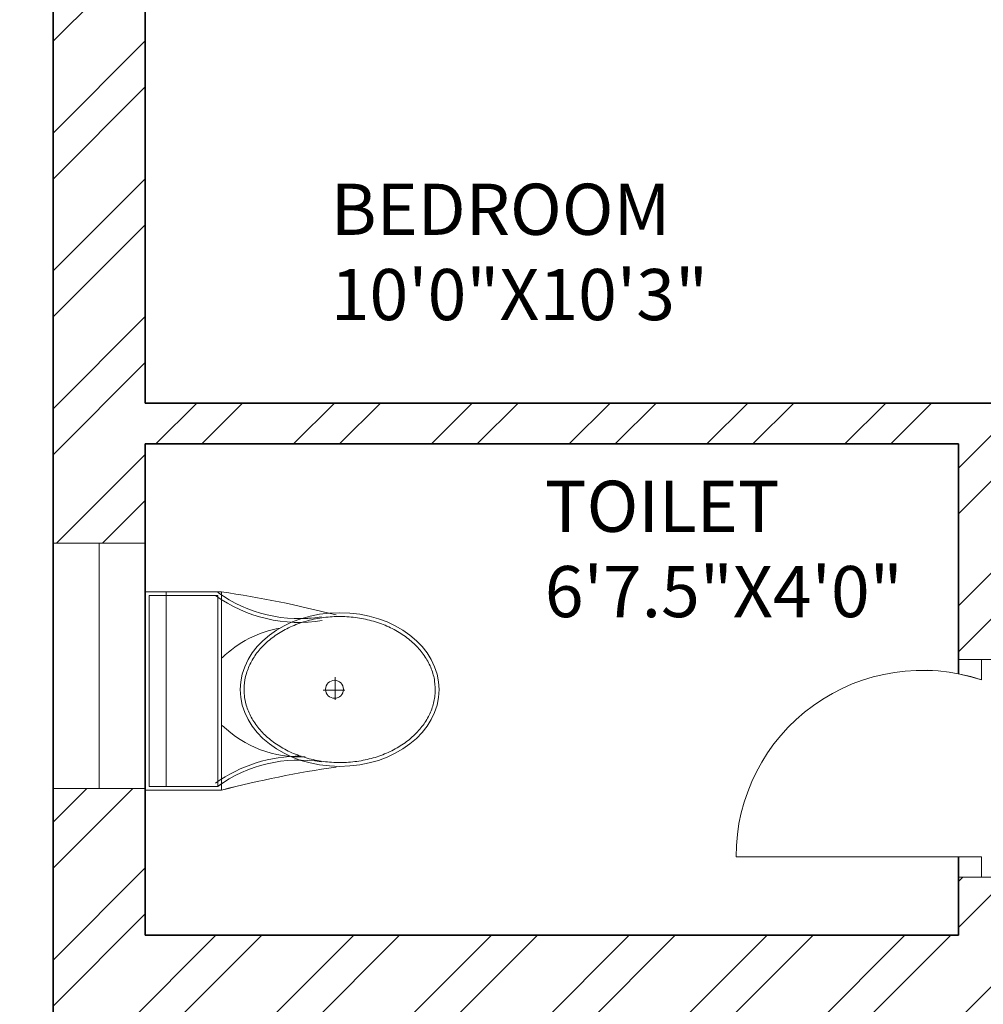
# Model space of a CAD drawing. Units: inches. Extents: x 2120 to 4013, y 1390 to 3019.
# Tile 7 of 59: x 2259 to 2354, y 1868 to 1964. Entities that reach past the tile are written whole.
import ezdxf

# ---------------------------------------------------------------- set-up
doc = ezdxf.new("R2010")
doc.units = ezdxf.units.IN
for name, color, linetype, lineweight in [('A-ANNO-DIMS', 2, 'Continuous', 18), ('A-AREA-IDEN', 7, 'Continuous', 18), ('A-DOOR', 3, 'Continuous', 18), ('A-FLOR-FIXT', 9, 'Continuous', 18), ('A-GLAZ', 4, 'Continuous', 18), ('A-WALL', 7, 'Continuous', 35), ('A-WALL-PATT', 252, 'Continuous', 13)]:
    doc.layers.add(name, color=color, linetype=linetype, lineweight=lineweight)
doc.styles.get("Standard").update_dxf_attribs({"font": 'arial.ttf'})
doc.dimstyles.get("Standard").update_dxf_attribs({"dimtxt": 0.18, "dimasz": 0.18, "dimexe": 0.18, "dimexo": 0.0625, "dimgap": 0.09, "dimtad": 0, "dimtih": 1, "dimtoh": 1, "dimdec": 4, "dimzin": 0, "dimdsep": 46, "dimtxsty": 'Standard', "dimcen": 0.09, "dimadec": 0, "dimazin": 0, "dimtfac": 1, "dimtdec": 4, "dimtofl": 0, "dimtmove": 0, "dimatfit": 3, "dimfxl": 1, "dimtolj": 1, "dimtzin": 0, "dimarcsym": 0})

# ---------------------------------------------------------------- blocks, each defined once
blk = doc.blocks.new('A$C31115884')
for p, q in [((257.5, 466.4), (257.5, 523.2)), ((283.1, 497.7), (223.4, 497.7)), ((0, 200), (0, 0)), ((520, 200), (0, 200)), ((10, 190), (10, 10)), ((510, 190), (10, 190)), ((510, 10), (510, 190)), ((520, 0), (520, 200)), ((510, 54.5), (0, 54.5)), ((10, 10), (510, 10)), ((0, 0), (520, 0))]:
    blk.add_line(p, q)
blk.add_circle((255.6, 496.4), 23.6)
for centre, radius, start, end in [((2777.7, -204.6), 2807, 165.4549, 171.7133), ((3237, 905), 2807, 188.2867, 194.5451), ((-294.5, 403.3), 364.7, 324.2091, 9.3499), ((-294.5, 403.3), 374.7, 324.2091, 9.3499), ((805.8, 403.3), 364.7, 170.6501, 215.7909), ((139.5, 406.2), 293.5, 315.8436, 2.6563), ((805.8, 403.3), 374.7, 179.2036, 215.7909), ((383.6, 406.2), 293.5, 190.2774, 224.1564)]:
    blk.add_arc(centre, radius, start, end)
blk.add_ellipse((256.2, 509.9), major_axis=(0, -260.7), ratio=0.772727)
blk.add_open_spline([(256.2, 259.2), (263.1, 259.2), (270, 259.7), (287.8, 262.3), (298.7, 265.1), (319.9, 273.1), (330.2, 278.4), (350.1, 291.1), (359.7, 298.7), (377.7, 315.9), (386.2, 325.5), (401.7, 346.6), (408.8, 358.1), (421.3, 382.5), (426.8, 395.5), (435.9, 422.4), (439.5, 436.4), (444.8, 465.1), (446.5, 479.7), (447.9, 509.2), (447.6, 524), (445, 553.3), (442.7, 567.8), (436.3, 596), (432.1, 609.7), (421.9, 636), (416, 648.6), (402.5, 672.1), (395, 683), (378.6, 703), (369.8, 712.1), (351.1, 728), (341.3, 734.8), (320.9, 746.2), (310.4, 750.7), (288.9, 757.3), (278, 759.4), (256, 761), (245, 760.6), (223.1, 757.2), (212.3, 754.3), (191.1, 746.1), (180.8, 740.7), (160.9, 727.8), (151.4, 720.1), (133.5, 702.7), (125.1, 693), (109.6, 671.7), (102.6, 660.2), (90.2, 635.7), (84.9, 622.7), (76, 595.6), (72.4, 581.6), (67.2, 552.9), (65.6, 538.2), (64.4, 508.8), (64.8, 494), (67.5, 464.7), (69.9, 450.2), (76.6, 422), (80.8, 408.3), (91.1, 382.2), (97.2, 369.7), (110.8, 346.3), (118.4, 335.4), (134.8, 315.6), (143.7, 306.7), (162.4, 290.9), (172.3, 284.2), (192.8, 273), (203.3, 268.6), (224.8, 262.2), (235.8, 260.2), (249.9, 259.3), (253, 259.2), (256.2, 259.2)], degree=3, knots=[0, 0, 0, 0, 0.110105, 0.110105, 0.285049, 0.285049, 0.459994, 0.459994, 0.634938, 0.634938, 0.809882, 0.809882, 0.984827, 0.984827, 1.159771, 1.159771, 1.334715, 1.334715, 1.50966, 1.50966, 1.684604, 1.684604, 1.859549, 1.859549, 2.034493, 2.034493, 2.209437, 2.209437, 2.384382, 2.384382, 2.559326, 2.559326, 2.73427, 2.73427, 2.909215, 2.909215, 3.084159, 3.084159, 3.259103, 3.259103, 3.434048, 3.434048, 3.608992, 3.608992, 3.783936, 3.783936, 3.958881, 3.958881, 4.133825, 4.133825, 4.30877, 4.30877, 4.483714, 4.483714, 4.658658, 4.658658, 4.833603, 4.833603, 5.008547, 5.008547, 5.183491, 5.183491, 5.358436, 5.358436, 5.53338, 5.53338, 5.708324, 5.708324, 5.883269, 5.883269, 6.058213, 6.058213, 6.233158, 6.233158, 6.283185, 6.283185, 6.283185, 6.283185])
blk = doc.blocks.new('DOOR-SWING-24IN-108p49DEG')
for p, q in [((21.75, 21.28), (26.25, 21.28)), ((26.25, 21.28), (24, 21.28)), ((24, 21.28), (24, 19.28)), ((24, 2), (0, 2)), ((24, 0), (24, 2)), ((26.25, 0), (21.75, 0)), ((21.75, 0), (24, 0))]:
    blk.add_line(p, q)
blk.add_arc((18.221, 2), 18.221, 71.50887, 180)
blk = doc.blocks.new('WIN-PLAN-24IN-03')
for p, q in [((9, 24), (0, 24)), ((0, 24), (4.5, 24)), ((4.5, 24), (4.5, 0)), ((9, 0), (0, 0)), ((4.5, 0), (9, 0))]:
    blk.add_line(p, q)
blk = doc.blocks.new('*D214')
at = {"layer": 'A-ANNO-DIMS', "color": 0, "lineweight": -2, "transparency": 16777216}
for p, q in [((2271.671, 2075.031), (2217.553, 2075.031)), ((2217.733, 2074.851), (2217.733, 1970.463)), ((2217.733, 1865.711), (2217.733, 1970.099)), ((2271.671, 1865.531), (2217.553, 1865.531))]:
    blk.add_line(p, q, dxfattribs=at)
at = {"layer": 'A-ANNO-DIMS', "color": 0, "transparency": 16777216}
for points in [[(2217.703, 2074.851), (2217.763, 2074.851), (2217.733, 2075.031)], [(2217.703, 1865.711), (2217.763, 1865.711), (2217.733, 1865.531)]]:
    blk.add_solid(points, dxfattribs=at)
at = {"layer": 'Defpoints', "color": 0, "transparency": 16777216}
for p in [(2217.733, 2075.031), (2271.733, 2075.031), (2271.733, 1865.531)]:
    blk.add_point(p, dxfattribs=at)
at = {"layer": 'A-ANNO-DIMS', "color": 0, "transparency": 16777216, "insert": (2217.733, 1970.281), "char_height": 0.18, "attachment_point": 5}
blk.add_mtext('\\A1;209.5', dxfattribs=at)

msp = doc.modelspace()

# ---------------------------------------------------------------- hatches: boundary and pattern name
at = {"layer": 'A-WALL-PATT'}
h = msp.add_hatch(dxfattribs=at)
h.set_pattern_fill('ANSI32', color=256)
h.paths.add_polyline_path([(2271.7331, 2343.531), (2283.3788, 2343.531), (2283.3788, 2348.031), (2283.3788, 2352.5306), (2262.7331, 2352.5306), (2262.7331, 2182.638), (2267.2331, 2182.638), (2271.7331, 2182.638), (2271.7331, 2219.031), (2391.7331, 2219.031), (2391.7331, 2214.189), (2393.9831, 2214.189), (2396.2331, 2214.189), (2396.2331, 2219.031), (2420.2331, 2219.031), (2420.2331, 2225.7535), (2417.2197, 2225.7535), (2415.7331, 2225.7535), (2415.7331, 2223.5306), (2271.7331, 2223.5306)])
h.paths.add_polyline_path([(2380.0942, 2352.5306), (2343.3788, 2352.5306), (2343.3788, 2343.531), (2363.2331, 2343.531), (2363.2331, 2288.8489), (2365.4831, 2288.8489), (2367.7331, 2288.8489), (2367.7331, 2343.531), (2380.0942, 2343.531)], flags=17)
h.paths.add_polyline_path([(2432.4339, 2352.5306), (2404.0943, 2352.5306), (2404.0943, 2343.531), (2415.7331, 2343.531), (2415.7331, 2264.0306), (2367.7331, 2264.0306), (2367.7331, 2266.4872), (2363.2331, 2266.4872), (2363.2331, 2259.531), (2367.7331, 2259.531), (2415.7331, 2259.531), (2415.7331, 2255.0658), (2420.2331, 2255.0658), (2420.2331, 2259.531), (2424.5717, 2259.531), (2424.5717, 2261.781), (2424.5717, 2264.0306), (2420.2331, 2264.0306), (2420.2331, 2343.531), (2432.4339, 2343.531)])
h.paths.add_polyline_path([(2508.9115, 2352.5306), (2456.4339, 2352.5306), (2456.4339, 2343.531), (2468.2331, 2343.531), (2468.2331, 2264.0306), (2448.0487, 2264.0306), (2448.0487, 2259.531), (2468.2331, 2259.531), (2468.2331, 2255.5496), (2472.7331, 2255.5496), (2472.7331, 2343.531), (2508.9115, 2343.531)])
h.paths.add_polyline_path([(2637.7331, 2352.5306), (2544.9116, 2352.5306), (2544.9116, 2343.531), (2589.7331, 2343.531), (2633.2331, 2343.531), (2637.7331, 2343.531)])
h.paths.add_polyline_path([(2594.2331, 2343.5306), (2589.7331, 2343.5306), (2589.7331, 2259.5306), (2589.7331, 2252.4915), (2591.9831, 2252.4915), (2594.2331, 2252.4915)])
h.paths.add_polyline_path([(2637.7331, 2223.5306), (2594.2331, 2223.5306), (2594.2331, 2230.1988), (2591.9831, 2230.1988), (2589.7331, 2230.1988), (2589.7331, 2223.5306), (2472.7331, 2223.5306), (2468.2331, 2223.5306), (2468.2331, 2219.031), (2628.7331, 2219.031), (2628.7331, 2138.031), (2637.7331, 2138.031)])
h.paths.add_polyline_path([(3822.6535, 2458.4402), (3874.9468, 2458.4402), (3874.9468, 2476.9866), (3822.6535, 2476.9866)], flags=9)
h.paths.add_polyline_path([(3834.6921, 2781.8174), (3935.9206, 2781.8174), (3935.9206, 2800.3638), (3834.6921, 2800.3638)], flags=9)
h.paths.add_polyline_path([(3832.2843, 2837.9683), (3884.5776, 2837.9683), (3884.5776, 2856.5146), (3832.2843, 2856.5146)], flags=9)
h.paths.add_polyline_path([(3830.9388, 2861.4782), (3956.8958, 2861.4782), (3956.8958, 2880.0245), (3830.9388, 2880.0245)], flags=9)
h.paths.add_polyline_path([(3870.6966, 2352.5752), (3887.9272, 2352.5752), (3887.9272, 2377.3037), (3870.6966, 2377.3037)], flags=9)
h.paths.add_polyline_path([(3289.2701, 2413.161), (3435.2223, 2413.161), (3435.2223, 2450.2538), (3289.2701, 2450.2538)], flags=9)
h.paths.add_polyline_path([(2487.6944, 2414.3601), (2637.8335, 2414.3601), (2637.8335, 2451.4528), (2487.6944, 2451.4528)], flags=9)
h.paths.add_polyline_path([(2567.3724, 1457.9199), (2815.296, 1457.9199), (2815.296, 1495.0127), (2567.3724, 1495.0127)], flags=9)
h.paths.add_polyline_path([(2655.3825, 2093.2363), (2685.9555, 2093.2363), (2685.9555, 2111.8937), (2655.3825, 2111.8937)], flags=9)
h.paths.add_polyline_path([(2543.9218, 1550.6671), (2587.8406, 1550.6671), (2587.8406, 1569.3244), (2543.9218, 1569.3244)], flags=9)
h.paths.add_polyline_path([(2905.1384, 1543.8113), (2949.0572, 1543.8113), (2949.0572, 1562.4686), (2905.1384, 1562.4686)], flags=9)
h.paths.add_polyline_path([(2736.4118, 1702.4736), (2784.2153, 1702.4736), (2784.2153, 1721.1309), (2736.4118, 1721.1309)], flags=9)
h.paths.add_polyline_path([(2912.8666, 1710.4168), (2951.707, 1710.4168), (2951.707, 1729.0741), (2912.8666, 1729.0741)], flags=9)
h.paths.add_polyline_path([(2923.5785, 1763.5038), (2959.7279, 1763.5038), (2959.7279, 1782.1611), (2923.5785, 1782.1611)], flags=9)
h.paths.add_polyline_path([(2925.2114, 1809.6137), (2967.1861, 1809.6137), (2967.1861, 1828.271), (2925.2114, 1828.271)], flags=9)
h.paths.add_polyline_path([(2996.2711, 1878.9003), (2996.2711, 1913.109), (2977.6138, 1913.109), (2977.6138, 1878.9003)], flags=9)
h.paths.add_polyline_path([(2883.0859, 1895.7192), (2927.1855, 1895.7192), (2927.1855, 1914.3766), (2883.0859, 1914.3766)], flags=9)
h.paths.add_polyline_path([(2787.3924, 1810.8013), (2841.0213, 1810.8013), (2841.0213, 1829.4587), (2787.3924, 1829.4587)], flags=9)
h.paths.add_polyline_path([(2775.6399, 2101.7395), (2829.2689, 2101.7395), (2829.2689, 2120.3968), (2775.6399, 2120.3968)], flags=9)
h.paths.add_polyline_path([(2913.0263, 2075.817), (2951.8667, 2075.817), (2951.8667, 2094.4744), (2913.0263, 2094.4744)], flags=9)
h.paths.add_polyline_path([(2929.966, 2133.3669), (2966.1154, 2133.3669), (2966.1154, 2152.0243), (2929.966, 2152.0243)], flags=9)
h.paths.add_polyline_path([(2932.7502, 2182.6088), (2968.8996, 2182.6088), (2968.8996, 2201.2662), (2932.7502, 2201.2662)], flags=9)
h.paths.add_polyline_path([(2996.0681, 2266.3173), (2996.0681, 2300.5261), (2977.4108, 2300.5261), (2977.4108, 2266.3173)], flags=9)
h.paths.add_polyline_path([(2885.1039, 2279.2186), (2929.2035, 2279.2186), (2929.2035, 2297.8759), (2885.1039, 2297.8759)], flags=9)
h.paths.add_polyline_path([(2735.7042, 2218.3197), (2783.5078, 2218.3197), (2783.5078, 2236.9771), (2735.7042, 2236.9771)], flags=9)
h.paths.add_polyline_path([(2635.6049, 2044.0085), (2648.9678, 2044.0085), (2648.9678, 2054.312), (2635.6049, 2054.312)], flags=9)
h.paths.add_polyline_path([(2714.0148, 1923.0473), (2727.3777, 1923.0473), (2727.3777, 1933.3508), (2714.0148, 1933.3508)], flags=9)
h.paths.add_polyline_path([(2709.0345, 1988.1628), (2722.3974, 1988.1628), (2722.3974, 1998.4663), (2709.0345, 1998.4663)], flags=9)
h.paths.add_polyline_path([(2592.8935, 1962.1763), (2606.2564, 1962.1763), (2606.2564, 1972.4799), (2592.8935, 1972.4799)], flags=9)
h.paths.add_polyline_path([(2618.3996, 1985.9724), (2644.1942, 1985.9724), (2644.1942, 1996.2759), (2618.3996, 1996.2759)], flags=9)
h.paths.add_polyline_path([(2601.279, 1920.5869), (2614.6419, 1920.5869), (2614.6419, 1930.8904), (2601.279, 1930.8904)], flags=9)
h.paths.add_polyline_path([(2692.3278, 1932.7645), (2704.5311, 1932.7645), (2704.5311, 1943.0681), (2692.3278, 1943.0681)], flags=9)
h.paths.add_polyline_path([(2311.122, 1672.7318), (2355.0408, 1672.7318), (2355.0408, 1691.3892), (2311.122, 1691.3892)], flags=9)
h.paths.add_polyline_path([(2456.2551, 1632.3198), (2492.4796, 1632.3198), (2492.4796, 1650.9772), (2456.2551, 1650.9772)], flags=9)
h.paths.add_polyline_path([(2401.0766, 1631.4793), (2437.301, 1631.4793), (2437.301, 1650.1367), (2401.0766, 1650.1367)], flags=9)
h.paths.add_polyline_path([(2546.7054, 1700.9235), (2594.509, 1700.9235), (2594.509, 1719.5809), (2546.7054, 1719.5809)], flags=9)
h.paths.add_polyline_path([(2445.4866, 1766.9937), (2497.5261, 1766.9937), (2497.5261, 1785.651), (2445.4866, 1785.651)], flags=9)
h.paths.add_polyline_path([(2287.9992, 1739.7675), (2326.8396, 1739.7675), (2326.8396, 1758.4248), (2287.9992, 1758.4248)], flags=9)
h.paths.add_polyline_path([(2458.5279, 1924.7607), (2510.5675, 1924.7607), (2510.5675, 1943.4181), (2458.5279, 1943.4181)], flags=9)
h.paths.add_polyline_path([(2309.2811, 1902.7642), (2345.4305, 1902.7642), (2345.4305, 1921.4215), (2309.2811, 1921.4215)], flags=9)
h.paths.add_polyline_path([(2490.7554, 2018.9392), (2530.7896, 2018.9392), (2530.7896, 2037.5965), (2490.7554, 2037.5965)], flags=9)
h.paths.add_polyline_path([(2402.143, 2024.7393), (2438.5414, 2024.7393), (2438.5414, 2043.3966), (2402.143, 2043.3966)], flags=9)
h.paths.add_polyline_path([(2287.856, 1931.7926), (2326.6964, 1931.7926), (2326.6964, 1950.4499), (2287.856, 1950.4499)], flags=9)
h.paths.add_polyline_path([(2281.7979, 2193.5771), (2320.6383, 2193.5771), (2320.6383, 2212.2344), (2281.7979, 2212.2344)], flags=25)
h.paths.add_polyline_path([(2484.0754, 2093.892), (2536.115, 2093.892), (2536.115, 2112.5494), (2484.0754, 2112.5494)], flags=9)
h.paths.add_polyline_path([(2624.7948, 2281.8639), (2624.7948, 2311.4137), (2606.1375, 2311.4137), (2606.1375, 2281.8639)], flags=9)
h.paths.add_polyline_path([(2507.5036, 2290.3639), (2541.934, 2290.3639), (2541.934, 2309.0212), (2507.5036, 2309.0212)], flags=9)
h.paths.add_polyline_path([(2423.1076, 2285.2202), (2459.332, 2285.2202), (2459.332, 2303.8776), (2423.1076, 2303.8776)], flags=9)
h.paths.add_polyline_path([(2374.5467, 2289.6272), (2410.7711, 2289.6272), (2410.7711, 2308.2846), (2374.5467, 2308.2846)], flags=25)
h.paths.add_polyline_path([(2277.4907, 2227.5651), (2316.3311, 2227.5651), (2316.3311, 2246.2224), (2277.4907, 2246.2224)], flags=25)
h.paths.add_polyline_path([(2655.3825, 2093.2367), (2685.9555, 2093.2367), (2685.9555, 2111.894), (2655.3825, 2111.894)], flags=9)
h.paths.add_polyline_path([(2543.9217, 1550.6674), (2587.8406, 1550.6674), (2587.8406, 1569.3247), (2543.9217, 1569.3247)], flags=9)
h.paths.add_polyline_path([(2905.1384, 1543.8116), (2949.0572, 1543.8116), (2949.0572, 1562.4689), (2905.1384, 1562.4689)], flags=9)
h.paths.add_polyline_path([(2736.4118, 1702.4739), (2784.2153, 1702.4739), (2784.2153, 1721.1312), (2736.4118, 1721.1312)], flags=9)
h.paths.add_polyline_path([(2912.8666, 1710.4171), (2951.707, 1710.4171), (2951.707, 1729.0744), (2912.8666, 1729.0744)], flags=9)
h.paths.add_polyline_path([(2923.5785, 1763.5041), (2959.7279, 1763.5041), (2959.7279, 1782.1614), (2923.5785, 1782.1614)], flags=9)
h.paths.add_polyline_path([(2925.2114, 1809.614), (2967.1861, 1809.614), (2967.1861, 1828.2713), (2925.2114, 1828.2713)], flags=9)
h.paths.add_polyline_path([(2996.2711, 1878.9006), (2996.2711, 1913.1094), (2977.6137, 1913.1094), (2977.6137, 1878.9006)], flags=9)
h.paths.add_polyline_path([(2883.0859, 1895.7195), (2927.1855, 1895.7195), (2927.1855, 1914.3769), (2883.0859, 1914.3769)], flags=9)
h.paths.add_polyline_path([(2787.3924, 1810.8016), (2841.0213, 1810.8016), (2841.0213, 1829.459), (2787.3924, 1829.459)], flags=9)
h.paths.add_polyline_path([(2775.6399, 2101.7398), (2829.2688, 2101.7398), (2829.2688, 2120.3971), (2775.6399, 2120.3971)], flags=9)
h.paths.add_polyline_path([(2913.0263, 2075.8173), (2951.8667, 2075.8173), (2951.8667, 2094.4747), (2913.0263, 2094.4747)], flags=9)
h.paths.add_polyline_path([(2929.966, 2133.3672), (2966.1154, 2133.3672), (2966.1154, 2152.0246), (2929.966, 2152.0246)], flags=9)
h.paths.add_polyline_path([(2932.7502, 2182.6091), (2968.8996, 2182.6091), (2968.8996, 2201.2665), (2932.7502, 2201.2665)], flags=9)
h.paths.add_polyline_path([(2996.0681, 2266.3176), (2996.0681, 2300.5264), (2977.4108, 2300.5264), (2977.4108, 2266.3176)], flags=9)
h.paths.add_polyline_path([(2885.1039, 2279.2189), (2929.2035, 2279.2189), (2929.2035, 2297.8762), (2885.1039, 2297.8762)], flags=9)
h.paths.add_polyline_path([(2735.7042, 2218.32), (2783.5078, 2218.32), (2783.5078, 2236.9774), (2735.7042, 2236.9774)], flags=9)
h.paths.add_polyline_path([(2635.6048, 2044.0088), (2648.9677, 2044.0088), (2648.9677, 2054.3123), (2635.6048, 2054.3123)], flags=9)
h.paths.add_polyline_path([(2714.0148, 1923.0476), (2727.3777, 1923.0476), (2727.3777, 1933.3511), (2714.0148, 1933.3511)], flags=9)
h.paths.add_polyline_path([(2709.0345, 1988.1631), (2722.3974, 1988.1631), (2722.3974, 1998.4666), (2709.0345, 1998.4666)], flags=9)
h.paths.add_polyline_path([(2592.8935, 1962.1766), (2606.2564, 1962.1766), (2606.2564, 1972.4802), (2592.8935, 1972.4802)], flags=9)
h.paths.add_polyline_path([(2618.3995, 1985.9727), (2644.1942, 1985.9727), (2644.1942, 1996.2762), (2618.3995, 1996.2762)], flags=9)
h.paths.add_polyline_path([(2601.279, 1920.5872), (2614.6419, 1920.5872), (2614.6419, 1930.8908), (2601.279, 1930.8908)], flags=9)
h.paths.add_polyline_path([(2692.3278, 1932.7648), (2704.5311, 1932.7648), (2704.5311, 1943.0684), (2692.3278, 1943.0684)], flags=9)
h.paths.add_polyline_path([(2311.122, 1672.7321), (2355.0408, 1672.7321), (2355.0408, 1691.3895), (2311.122, 1691.3895)], flags=9)
h.paths.add_polyline_path([(2456.2551, 1632.3201), (2492.4795, 1632.3201), (2492.4795, 1650.9775), (2456.2551, 1650.9775)], flags=9)
h.paths.add_polyline_path([(2401.0766, 1631.4796), (2437.301, 1631.4796), (2437.301, 1650.137), (2401.0766, 1650.137)], flags=9)
h.paths.add_polyline_path([(2546.7054, 1700.9238), (2594.509, 1700.9238), (2594.509, 1719.5812), (2546.7054, 1719.5812)], flags=9)
h.paths.add_polyline_path([(2445.4866, 1766.994), (2497.5261, 1766.994), (2497.5261, 1785.6513), (2445.4866, 1785.6513)], flags=9)
h.paths.add_polyline_path([(2287.9992, 1739.7678), (2326.8396, 1739.7678), (2326.8396, 1758.4251), (2287.9992, 1758.4251)], flags=9)
h.paths.add_polyline_path([(2458.5279, 1924.7611), (2510.5675, 1924.7611), (2510.5675, 1943.4184), (2458.5279, 1943.4184)], flags=9)
h.paths.add_polyline_path([(2309.2811, 1902.7645), (2345.4305, 1902.7645), (2345.4305, 1921.4218), (2309.2811, 1921.4218)], flags=9)
h.paths.add_polyline_path([(2490.7554, 2018.9395), (2530.7895, 2018.9395), (2530.7895, 2037.5968), (2490.7554, 2037.5968)], flags=9)
h.paths.add_polyline_path([(2402.143, 2024.7396), (2438.5413, 2024.7396), (2438.5413, 2043.3969), (2402.143, 2043.3969)], flags=9)
h.paths.add_polyline_path([(2287.856, 1931.7929), (2326.6964, 1931.7929), (2326.6964, 1950.4502), (2287.856, 1950.4502)], flags=9)
h.paths.add_polyline_path([(2281.7979, 2193.5774), (2320.6383, 2193.5774), (2320.6383, 2212.2347), (2281.7979, 2212.2347)], flags=25)
h.paths.add_polyline_path([(2484.0754, 2093.8924), (2536.115, 2093.8924), (2536.115, 2112.5497), (2484.0754, 2112.5497)], flags=9)
h.paths.add_polyline_path([(2624.7948, 2281.8642), (2624.7948, 2311.414), (2606.1374, 2311.414), (2606.1374, 2281.8642)], flags=9)
h.paths.add_polyline_path([(2507.5035, 2290.3642), (2541.934, 2290.3642), (2541.934, 2309.0215), (2507.5035, 2309.0215)], flags=9)
h.paths.add_polyline_path([(2423.1075, 2285.2205), (2459.332, 2285.2205), (2459.332, 2303.8779), (2423.1075, 2303.8779)], flags=9)
h.paths.add_polyline_path([(2374.5467, 2289.6275), (2410.7711, 2289.6275), (2410.7711, 2308.2849), (2374.5467, 2308.2849)], flags=25)
h.paths.add_polyline_path([(2277.4907, 2227.5654), (2316.3311, 2227.5654), (2316.3311, 2246.2227), (2277.4907, 2246.2227)], flags=25)
h = msp.add_hatch(dxfattribs=at)
h.set_pattern_fill('ANSI32', color=256)
h.paths.add_polyline_path([(2271.7331, 1980.389), (2262.7331, 1980.389), (2262.7331, 1912.8434), (2267.2331, 1912.8434), (2271.7331, 1912.8434), (2271.7331, 1922.531), (2351.2331, 1922.531), (2351.2331, 1901.4728), (2355.7331, 1901.4728), (2355.7331, 1922.531), (2357.9815, 1922.531), (2357.9815, 1926.5306), (2271.7331, 1926.5306)])
h.paths.add_polyline_path([(2589.2331, 1949.1622), (2584.7331, 1949.1622), (2580.2331, 1949.1622), (2580.2331, 1874.5306), (2355.7331, 1874.5306), (2355.7331, 1880.1922), (2351.2331, 1880.1922), (2351.2331, 1874.5306), (2271.7331, 1874.5306), (2271.7331, 1888.8431), (2262.7331, 1888.8431), (2262.7331, 1842.2909), (2267.2331, 1842.2909), (2271.7331, 1842.2909), (2271.7331, 1865.531), (2415.7331, 1865.531), (2415.7331, 1779.7286), (2420.2331, 1779.7286), (2420.2331, 1865.531), (2589.2331, 1865.531)])
h.paths.add_polyline_path([(2271.7331, 1782.2906), (2262.7331, 1782.2906), (2262.7331, 1711.4639), (2267.2331, 1711.4639), (2271.7331, 1711.4639), (2271.7331, 1738.031), (2420.2331, 1738.031), (2420.2331, 1742.531), (2420.2331, 1747.3376), (2417.9831, 1747.3376), (2415.7331, 1747.3376), (2415.7331, 1742.5306), (2271.7331, 1742.5306)])
h.paths.add_polyline_path([(2271.7331, 1627.031), (2362.3957, 1627.031), (2362.3957, 1629.281), (2362.3957, 1631.5306), (2271.7331, 1631.5306), (2271.7331, 1675.4636), (2262.7331, 1675.4636), (2262.7331, 1581.531), (2405.3032, 1581.531), (2405.3032, 1586.031), (2405.3032, 1590.5306), (2396.2331, 1590.5306), (2396.2331, 1691.4513), (2418.7206, 1691.4513), (2418.7206, 1695.951), (2396.2331, 1695.951), (2391.7331, 1695.951), (2391.7331, 1631.5306), (2386.7425, 1631.5306), (2386.7425, 1629.2806), (2386.7425, 1627.031), (2391.7331, 1627.031), (2391.7331, 1586.1709), (2271.7331, 1586.1709)])
h.paths.add_polyline_path([(2459.6703, 1590.5306), (2429.3032, 1590.5306), (2429.3032, 1581.531), (2459.6703, 1581.531), (2459.6703, 1586.031)])
h.paths.add_polyline_path([(2501.2331, 1590.531), (2501.2331, 1665.0195), (2498.9831, 1665.0195), (2496.7331, 1665.0195), (2496.7331, 1590.5306), (2483.8201, 1590.5306), (2483.8201, 1590.1579), (2483.6704, 1590.1579), (2483.6704, 1581.531), (2505.0196, 1581.531), (2505.0196, 1583.781), (2505.0196, 1586.0306), (2501.2331, 1586.0306)])
h.paths.add_polyline_path([(2544.1361, 1583.781), (2544.1361, 1586.0306), (2527.1368, 1586.0306), (2527.1368, 1583.7806), (2527.1368, 1581.531), (2544.1361, 1581.531)])
h.paths.add_polyline_path([(3822.6535, 2458.4402), (3874.9468, 2458.4402), (3874.9468, 2476.9866), (3822.6535, 2476.9866)], flags=9)
h.paths.add_polyline_path([(3834.6921, 2781.8174), (3935.9206, 2781.8174), (3935.9206, 2800.3638), (3834.6921, 2800.3638)], flags=9)
h.paths.add_polyline_path([(3832.2843, 2837.9683), (3884.5776, 2837.9683), (3884.5776, 2856.5146), (3832.2843, 2856.5146)], flags=9)
h.paths.add_polyline_path([(3830.9388, 2861.4782), (3956.8958, 2861.4782), (3956.8958, 2880.0245), (3830.9388, 2880.0245)], flags=9)
h.paths.add_polyline_path([(3870.6966, 2352.5752), (3887.9272, 2352.5752), (3887.9272, 2377.3037), (3870.6966, 2377.3037)], flags=9)
h.paths.add_polyline_path([(3289.2701, 2413.161), (3435.2223, 2413.161), (3435.2223, 2450.2538), (3289.2701, 2450.2538)], flags=9)
h.paths.add_polyline_path([(2487.6944, 2414.3601), (2637.8335, 2414.3601), (2637.8335, 2451.4528), (2487.6944, 2451.4528)], flags=9)
h.paths.add_polyline_path([(2567.3724, 1457.9199), (2815.296, 1457.9199), (2815.296, 1495.0127), (2567.3724, 1495.0127)], flags=9)
h.paths.add_polyline_path([(2655.3825, 2093.2363), (2685.9555, 2093.2363), (2685.9555, 2111.8937), (2655.3825, 2111.8937)], flags=9)
h.paths.add_polyline_path([(2543.9218, 1550.6671), (2587.8406, 1550.6671), (2587.8406, 1569.3244), (2543.9218, 1569.3244)], flags=9)
h.paths.add_polyline_path([(2905.1384, 1543.8113), (2949.0572, 1543.8113), (2949.0572, 1562.4686), (2905.1384, 1562.4686)], flags=9)
h.paths.add_polyline_path([(2736.4118, 1702.4736), (2784.2153, 1702.4736), (2784.2153, 1721.1309), (2736.4118, 1721.1309)], flags=9)
h.paths.add_polyline_path([(2912.8666, 1710.4168), (2951.707, 1710.4168), (2951.707, 1729.0741), (2912.8666, 1729.0741)], flags=9)
h.paths.add_polyline_path([(2923.5785, 1763.5038), (2959.7279, 1763.5038), (2959.7279, 1782.1611), (2923.5785, 1782.1611)], flags=9)
h.paths.add_polyline_path([(2925.2114, 1809.6137), (2967.1861, 1809.6137), (2967.1861, 1828.271), (2925.2114, 1828.271)], flags=9)
h.paths.add_polyline_path([(2996.2711, 1878.9003), (2996.2711, 1913.109), (2977.6138, 1913.109), (2977.6138, 1878.9003)], flags=9)
h.paths.add_polyline_path([(2883.0859, 1895.7192), (2927.1855, 1895.7192), (2927.1855, 1914.3766), (2883.0859, 1914.3766)], flags=9)
h.paths.add_polyline_path([(2787.3924, 1810.8013), (2841.0213, 1810.8013), (2841.0213, 1829.4587), (2787.3924, 1829.4587)], flags=9)
h.paths.add_polyline_path([(2775.6399, 2101.7395), (2829.2689, 2101.7395), (2829.2689, 2120.3968), (2775.6399, 2120.3968)], flags=9)
h.paths.add_polyline_path([(2913.0263, 2075.817), (2951.8667, 2075.817), (2951.8667, 2094.4744), (2913.0263, 2094.4744)], flags=9)
h.paths.add_polyline_path([(2929.966, 2133.3669), (2966.1154, 2133.3669), (2966.1154, 2152.0243), (2929.966, 2152.0243)], flags=9)
h.paths.add_polyline_path([(2932.7502, 2182.6088), (2968.8996, 2182.6088), (2968.8996, 2201.2662), (2932.7502, 2201.2662)], flags=9)
h.paths.add_polyline_path([(2996.0681, 2266.3173), (2996.0681, 2300.5261), (2977.4108, 2300.5261), (2977.4108, 2266.3173)], flags=9)
h.paths.add_polyline_path([(2885.1039, 2279.2186), (2929.2035, 2279.2186), (2929.2035, 2297.8759), (2885.1039, 2297.8759)], flags=9)
h.paths.add_polyline_path([(2735.7042, 2218.3197), (2783.5078, 2218.3197), (2783.5078, 2236.9771), (2735.7042, 2236.9771)], flags=9)
h.paths.add_polyline_path([(2635.6049, 2044.0085), (2648.9678, 2044.0085), (2648.9678, 2054.312), (2635.6049, 2054.312)], flags=9)
h.paths.add_polyline_path([(2714.0148, 1923.0473), (2727.3777, 1923.0473), (2727.3777, 1933.3508), (2714.0148, 1933.3508)], flags=9)
h.paths.add_polyline_path([(2709.0345, 1988.1628), (2722.3974, 1988.1628), (2722.3974, 1998.4663), (2709.0345, 1998.4663)], flags=9)
h.paths.add_polyline_path([(2592.8935, 1962.1763), (2606.2564, 1962.1763), (2606.2564, 1972.4799), (2592.8935, 1972.4799)], flags=9)
h.paths.add_polyline_path([(2618.3996, 1985.9724), (2644.1942, 1985.9724), (2644.1942, 1996.2759), (2618.3996, 1996.2759)], flags=9)
h.paths.add_polyline_path([(2601.279, 1920.5869), (2614.6419, 1920.5869), (2614.6419, 1930.8904), (2601.279, 1930.8904)], flags=9)
h.paths.add_polyline_path([(2692.3278, 1932.7645), (2704.5311, 1932.7645), (2704.5311, 1943.0681), (2692.3278, 1943.0681)], flags=9)
h.paths.add_polyline_path([(2311.122, 1672.7318), (2355.0408, 1672.7318), (2355.0408, 1691.3892), (2311.122, 1691.3892)], flags=25)
h.paths.add_polyline_path([(2456.2551, 1632.3198), (2492.4796, 1632.3198), (2492.4796, 1650.9772), (2456.2551, 1650.9772)], flags=9)
h.paths.add_polyline_path([(2401.0766, 1631.4793), (2437.301, 1631.4793), (2437.301, 1650.1367), (2401.0766, 1650.1367)], flags=9)
h.paths.add_polyline_path([(2546.7054, 1700.9235), (2594.509, 1700.9235), (2594.509, 1719.5809), (2546.7054, 1719.5809)], flags=9)
h.paths.add_polyline_path([(2445.4866, 1766.9937), (2497.5261, 1766.9937), (2497.5261, 1785.651), (2445.4866, 1785.651)], flags=9)
h.paths.add_polyline_path([(2287.9992, 1739.7675), (2326.8396, 1739.7675), (2326.8396, 1758.4248), (2287.9992, 1758.4248)], flags=24)
h.paths.add_polyline_path([(2458.5279, 1924.7607), (2510.5675, 1924.7607), (2510.5675, 1943.4181), (2458.5279, 1943.4181)], flags=25)
h.paths.add_polyline_path([(2309.2811, 1902.7642), (2345.4305, 1902.7642), (2345.4305, 1921.4215), (2309.2811, 1921.4215)], flags=25)
h.paths.add_polyline_path([(2490.7554, 2018.9392), (2530.7896, 2018.9392), (2530.7896, 2037.5965), (2490.7554, 2037.5965)], flags=9)
h.paths.add_polyline_path([(2402.143, 2024.7393), (2438.5414, 2024.7393), (2438.5414, 2043.3966), (2402.143, 2043.3966)], flags=9)
h.paths.add_polyline_path([(2287.856, 1931.7926), (2326.6964, 1931.7926), (2326.6964, 1950.4499), (2287.856, 1950.4499)], flags=25)
h.paths.add_polyline_path([(2281.7979, 2193.5771), (2320.6383, 2193.5771), (2320.6383, 2212.2344), (2281.7979, 2212.2344)], flags=9)
h.paths.add_polyline_path([(2484.0754, 2093.892), (2536.115, 2093.892), (2536.115, 2112.5494), (2484.0754, 2112.5494)], flags=9)
h.paths.add_polyline_path([(2624.7948, 2281.8639), (2624.7948, 2311.4137), (2606.1375, 2311.4137), (2606.1375, 2281.8639)], flags=9)
h.paths.add_polyline_path([(2507.5036, 2290.3639), (2541.934, 2290.3639), (2541.934, 2309.0212), (2507.5036, 2309.0212)], flags=9)
h.paths.add_polyline_path([(2423.1076, 2285.2202), (2459.332, 2285.2202), (2459.332, 2303.8776), (2423.1076, 2303.8776)], flags=9)
h.paths.add_polyline_path([(2374.5467, 2289.6272), (2410.7711, 2289.6272), (2410.7711, 2308.2846), (2374.5467, 2308.2846)], flags=9)
h.paths.add_polyline_path([(2277.4907, 2227.5651), (2316.3311, 2227.5651), (2316.3311, 2246.2224), (2277.4907, 2246.2224)], flags=9)
h.paths.add_polyline_path([(2655.3825, 2093.2367), (2685.9555, 2093.2367), (2685.9555, 2111.894), (2655.3825, 2111.894)], flags=9)
h.paths.add_polyline_path([(2543.9217, 1550.6674), (2587.8406, 1550.6674), (2587.8406, 1569.3247), (2543.9217, 1569.3247)], flags=9)
h.paths.add_polyline_path([(2905.1384, 1543.8116), (2949.0572, 1543.8116), (2949.0572, 1562.4689), (2905.1384, 1562.4689)], flags=9)
h.paths.add_polyline_path([(2736.4118, 1702.4739), (2784.2153, 1702.4739), (2784.2153, 1721.1312), (2736.4118, 1721.1312)], flags=9)
h.paths.add_polyline_path([(2912.8666, 1710.4171), (2951.707, 1710.4171), (2951.707, 1729.0744), (2912.8666, 1729.0744)], flags=9)
h.paths.add_polyline_path([(2923.5785, 1763.5041), (2959.7279, 1763.5041), (2959.7279, 1782.1614), (2923.5785, 1782.1614)], flags=9)
h.paths.add_polyline_path([(2925.2114, 1809.614), (2967.1861, 1809.614), (2967.1861, 1828.2713), (2925.2114, 1828.2713)], flags=9)
h.paths.add_polyline_path([(2996.2711, 1878.9006), (2996.2711, 1913.1094), (2977.6137, 1913.1094), (2977.6137, 1878.9006)], flags=9)
h.paths.add_polyline_path([(2883.0859, 1895.7195), (2927.1855, 1895.7195), (2927.1855, 1914.3769), (2883.0859, 1914.3769)], flags=9)
h.paths.add_polyline_path([(2787.3924, 1810.8016), (2841.0213, 1810.8016), (2841.0213, 1829.459), (2787.3924, 1829.459)], flags=9)
h.paths.add_polyline_path([(2775.6399, 2101.7398), (2829.2688, 2101.7398), (2829.2688, 2120.3971), (2775.6399, 2120.3971)], flags=9)
h.paths.add_polyline_path([(2913.0263, 2075.8173), (2951.8667, 2075.8173), (2951.8667, 2094.4747), (2913.0263, 2094.4747)], flags=9)
h.paths.add_polyline_path([(2929.966, 2133.3672), (2966.1154, 2133.3672), (2966.1154, 2152.0246), (2929.966, 2152.0246)], flags=9)
h.paths.add_polyline_path([(2932.7502, 2182.6091), (2968.8996, 2182.6091), (2968.8996, 2201.2665), (2932.7502, 2201.2665)], flags=9)
h.paths.add_polyline_path([(2996.0681, 2266.3176), (2996.0681, 2300.5264), (2977.4108, 2300.5264), (2977.4108, 2266.3176)], flags=9)
h.paths.add_polyline_path([(2885.1039, 2279.2189), (2929.2035, 2279.2189), (2929.2035, 2297.8762), (2885.1039, 2297.8762)], flags=9)
h.paths.add_polyline_path([(2735.7042, 2218.32), (2783.5078, 2218.32), (2783.5078, 2236.9774), (2735.7042, 2236.9774)], flags=9)
h.paths.add_polyline_path([(2635.6048, 2044.0088), (2648.9677, 2044.0088), (2648.9677, 2054.3123), (2635.6048, 2054.3123)], flags=9)
h.paths.add_polyline_path([(2714.0148, 1923.0476), (2727.3777, 1923.0476), (2727.3777, 1933.3511), (2714.0148, 1933.3511)], flags=9)
h.paths.add_polyline_path([(2709.0345, 1988.1631), (2722.3974, 1988.1631), (2722.3974, 1998.4666), (2709.0345, 1998.4666)], flags=9)
h.paths.add_polyline_path([(2592.8935, 1962.1766), (2606.2564, 1962.1766), (2606.2564, 1972.4802), (2592.8935, 1972.4802)], flags=9)
h.paths.add_polyline_path([(2618.3995, 1985.9727), (2644.1942, 1985.9727), (2644.1942, 1996.2762), (2618.3995, 1996.2762)], flags=9)
h.paths.add_polyline_path([(2601.279, 1920.5872), (2614.6419, 1920.5872), (2614.6419, 1930.8908), (2601.279, 1930.8908)], flags=9)
h.paths.add_polyline_path([(2692.3278, 1932.7648), (2704.5311, 1932.7648), (2704.5311, 1943.0684), (2692.3278, 1943.0684)], flags=9)
h.paths.add_polyline_path([(2311.122, 1672.7321), (2355.0408, 1672.7321), (2355.0408, 1691.3895), (2311.122, 1691.3895)], flags=25)
h.paths.add_polyline_path([(2456.2551, 1632.3201), (2492.4795, 1632.3201), (2492.4795, 1650.9775), (2456.2551, 1650.9775)], flags=9)
h.paths.add_polyline_path([(2401.0766, 1631.4796), (2437.301, 1631.4796), (2437.301, 1650.137), (2401.0766, 1650.137)], flags=9)
h.paths.add_polyline_path([(2546.7054, 1700.9238), (2594.509, 1700.9238), (2594.509, 1719.5812), (2546.7054, 1719.5812)], flags=9)
h.paths.add_polyline_path([(2445.4866, 1766.994), (2497.5261, 1766.994), (2497.5261, 1785.6513), (2445.4866, 1785.6513)], flags=9)
h.paths.add_polyline_path([(2287.9992, 1739.7678), (2326.8396, 1739.7678), (2326.8396, 1758.4251), (2287.9992, 1758.4251)], flags=24)
h.paths.add_polyline_path([(2458.5279, 1924.7611), (2510.5675, 1924.7611), (2510.5675, 1943.4184), (2458.5279, 1943.4184)], flags=25)
h.paths.add_polyline_path([(2309.2811, 1902.7645), (2345.4305, 1902.7645), (2345.4305, 1921.4218), (2309.2811, 1921.4218)], flags=25)
h.paths.add_polyline_path([(2490.7554, 2018.9395), (2530.7895, 2018.9395), (2530.7895, 2037.5968), (2490.7554, 2037.5968)], flags=9)
h.paths.add_polyline_path([(2402.143, 2024.7396), (2438.5413, 2024.7396), (2438.5413, 2043.3969), (2402.143, 2043.3969)], flags=9)
h.paths.add_polyline_path([(2287.856, 1931.7929), (2326.6964, 1931.7929), (2326.6964, 1950.4502), (2287.856, 1950.4502)], flags=25)
h.paths.add_polyline_path([(2281.7979, 2193.5774), (2320.6383, 2193.5774), (2320.6383, 2212.2347), (2281.7979, 2212.2347)], flags=9)
h.paths.add_polyline_path([(2484.0754, 2093.8924), (2536.115, 2093.8924), (2536.115, 2112.5497), (2484.0754, 2112.5497)], flags=9)
h.paths.add_polyline_path([(2624.7948, 2281.8642), (2624.7948, 2311.414), (2606.1374, 2311.414), (2606.1374, 2281.8642)], flags=9)
h.paths.add_polyline_path([(2507.5035, 2290.3642), (2541.934, 2290.3642), (2541.934, 2309.0215), (2507.5035, 2309.0215)], flags=9)
h.paths.add_polyline_path([(2423.1075, 2285.2205), (2459.332, 2285.2205), (2459.332, 2303.8779), (2423.1075, 2303.8779)], flags=9)
h.paths.add_polyline_path([(2374.5467, 2289.6275), (2410.7711, 2289.6275), (2410.7711, 2308.2849), (2374.5467, 2308.2849)], flags=9)
h.paths.add_polyline_path([(2277.4907, 2227.5654), (2316.3311, 2227.5654), (2316.3311, 2246.2227), (2277.4907, 2246.2227)], flags=9)

# ---------------------------------------------------------------- linework, layer by layer
at = {"layer": 'A-WALL'}
for p, q in [((2262.7331, 2352.531), (2262.7331, 1581.531)), ((2262.7331, 2352.5306), (2262.7331, 1581.5306)), ((2271.7331, 2070.531), (2271.7331, 1926.531)), ((2271.7331, 2070.5306), (2271.7331, 1926.5306)), ((2271.7331, 1926.531), (2359.434, 1926.531)), ((2271.7331, 1926.5306), (2359.434, 1926.5306)), ((2271.7331, 1922.531), (2351.2331, 1922.531)), ((2271.7331, 1922.531), (2271.7331, 1874.531)), ((2271.7331, 1922.5306), (2351.2331, 1922.5306)), ((2271.7331, 1922.5306), (2271.7331, 1874.5306)), ((2351.2331, 1900.0685), (2351.2331, 1922.531)), ((2351.2331, 1900.0682), (2351.2331, 1922.5306)), ((2351.2331, 1874.531), (2351.2331, 1882.1925)), ((2351.2331, 1874.5306), (2351.2331, 1882.1922)), ((2271.7331, 1874.531), (2351.2331, 1874.531)), ((2271.7331, 1874.531), (2351.2331, 1874.531)), ((2271.7331, 1874.5306), (2351.2331, 1874.5306)), ((2271.7331, 1874.5306), (2351.2331, 1874.5306))]:
    msp.add_line(p, q, dxfattribs=at)

# ---------------------------------------------------------------- block references
at = {"layer": 'A-DOOR'}
for p in [(2329.4831, 1880.1925), (2329.4831, 1880.1922)]:
    msp.add_blockref('DOOR-SWING-24IN-108p49DEG', p, dxfattribs=at)
at = {"layer": 'A-FLOR-FIXT', "xscale": 0.0372717239612423, "yscale": 0.0372717239612423, "zscale": 0.0372717239612423, "rotation": 270}
for p in [(2271.7331, 1908.0784), (2271.7331, 1908.0781)]:
    msp.add_blockref('A$C31115884', p, dxfattribs=at)
at = {"layer": 'A-GLAZ'}
for p in [(2262.7331, 1888.8434), (2262.7331, 1888.8431)]:
    msp.add_blockref('WIN-PLAN-24IN-03', p, dxfattribs=at)

# ---------------------------------------------------------------- texts
at = {"layer": 'A-AREA-IDEN', "char_height": 5, "attachment_point": 1}
for s, width, insert in [('BEDROOM\\P10\'0"X10\'3"', 122.863072, (2289.8666, 1947.9656)), ('BEDROOM\\P10\'0"X10\'3"', 122.863072, (2289.8666, 1947.9653)), ('TOILET\\P6\'7.5"X4\'0"', 111.070309, (2310.7937, 1918.9372)), ('TOILET\\P6\'7.5"X4\'0"', 111.070309, (2310.7937, 1918.9369))]:
    msp.add_mtext_dynamic_manual_height_columns(s, width=width, gutter_width=12.5, heights=[0], dxfattribs=dict(at, insert=insert))

# ---------------------------------------------------------------- dimensions: what is measured, and where the dimension line sits
at = {"layer": 'A-ANNO-DIMS'}
dim = msp.add_linear_dim(base=(2217.7331, 2075.031), p1=(2271.7331, 1865.531), p2=(2271.7331, 2075.031), angle=90, dimstyle='Standard', override={"dimdec": 1, "dimlfac": 1, "dimrnd": 0, "dimzin": 0, "dimdsep": 46, "dimlunit": 2}, dxfattribs=at)
dim.commit()
dim.dimension.update_dxf_attribs({"geometry": '*D214', "text_midpoint": (2217.7331, 1970.281)})

doc.saveas('drawing.dxf')
